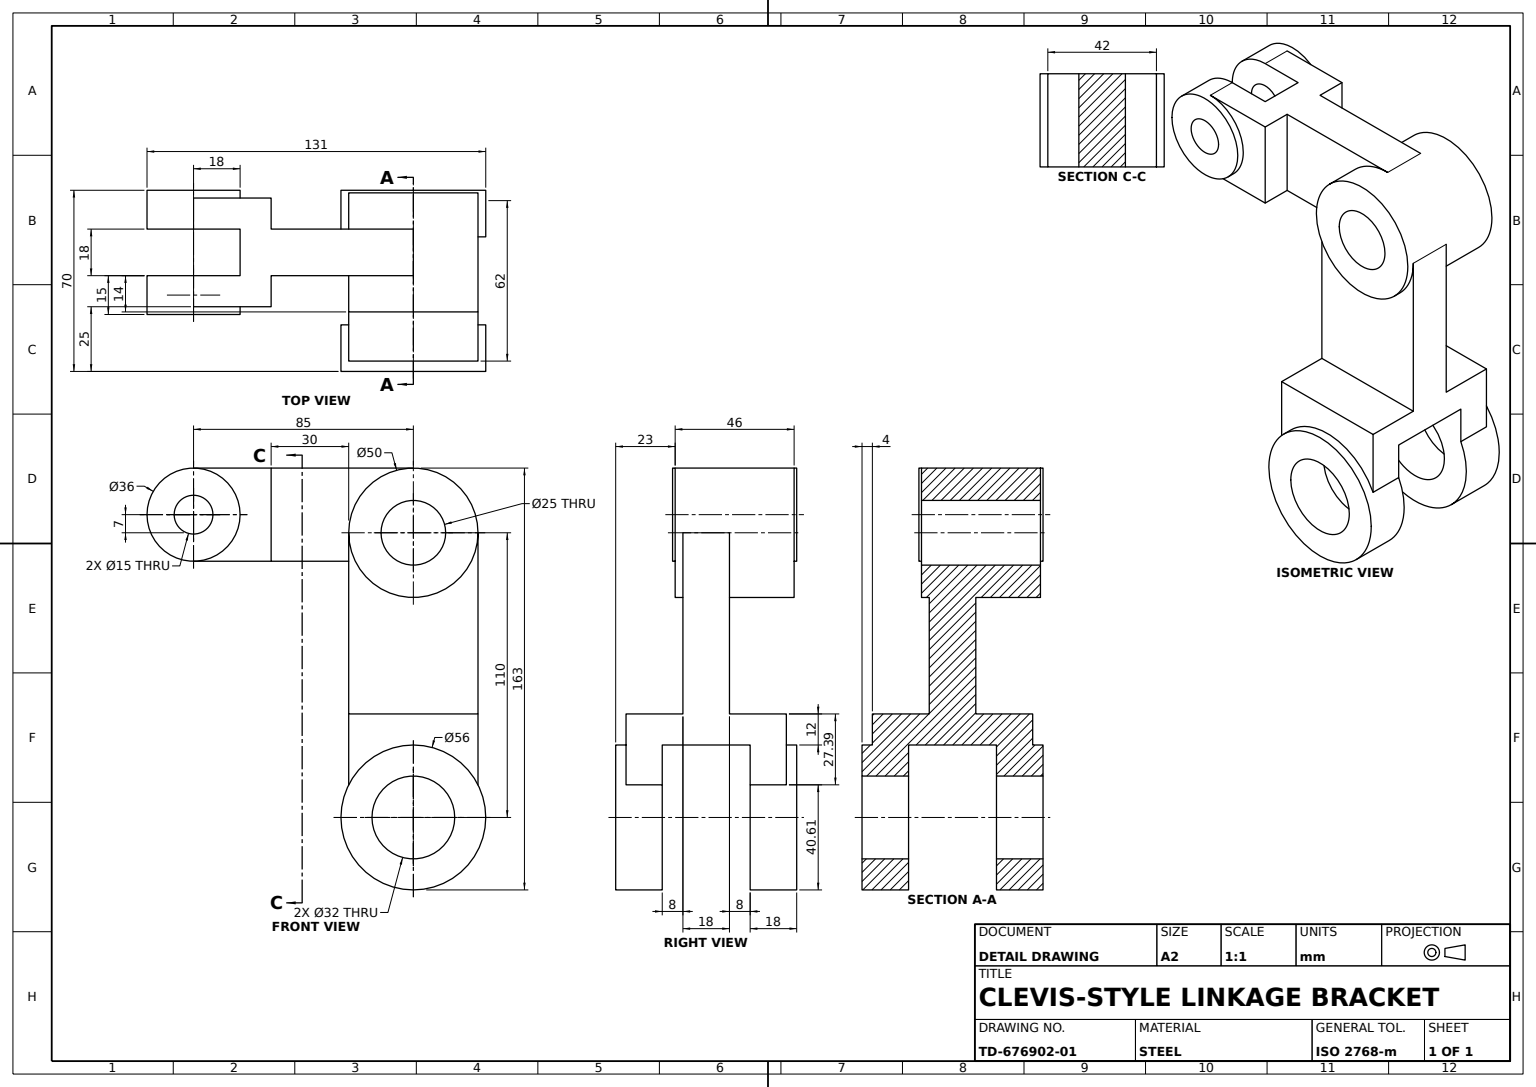
from build123d import *

# Parameters (mm, degrees)
LOWER_HUB_A_SKETCH_R        = 28
LOWER_HUB_A_56_DEPTH        = 18
LOWER_HUB_B_SKETCH_R        = 28
LOWER_HUB_B_56_DEPTH        = 18
LOWER_FORK_BLOCK_DEPTH      = 48
LOWER_FORK_BLOCK_DEPTH_BACK = 14
LOWER_FORK_SLOT_SKETCH_W    = 34
LOWER_FORK_SLOT_SKETCH_H    = 15.390479787
LOWER_FORK_SLOT_DEPTH       = 65
VERTICAL_ARM_DEPTH          = 50
UPPER_HUB_DEPTH             = 3
UPPER_HUB_DEPTH_BACK        = 43
UPPER_HUB_SKETCH_R          = 25
UPPER_FORK_ARM_DEPTH        = 36
FORK_EYE_A_SKETCH_R         = 18
FORK_EYE_A_36_DEPTH         = 15
FORK_START                  = -15
FORK_EYE_B_SKETCH_R         = 18
FORK_EYE_B_DEPTH            = 15
LOWER_PIVOT_BORE_SKETCH_R   = 16
LOWER_PIVOT_BORE_32_DEPTH   = 132
UPPER_HUB_BORE_SKETCH_R     = 12.5
UPPER_HUB_BORE_25_DEPTH     = 132
FORK_EYE_BORE_SKETCH_R      = 7.5
FORK_EYE_BORE_15_DEPTH      = 132


with BuildPart() as part:
    # Lower Hub A Sketch → Lower Hub A Ø56 (new body)
    with BuildSketch(Plane(origin=(0, 0, 0), x_dir=(0, 0, -1), z_dir=(1, 0, 0))):
        Circle(LOWER_HUB_A_SKETCH_R)
    extrude(amount=-LOWER_HUB_A_56_DEPTH)



with BuildPart() as body_2:
    # Lower Hub B Sketch → Lower Hub B Ø56 (new body)
    with BuildSketch(Plane.ZY.offset(52)):
        with Locations(Location((0, 0, 0), (0, 0, 180))):
            Circle(LOWER_HUB_B_SKETCH_R)
    extrude(amount=LOWER_HUB_B_56_DEPTH)


with BuildPart() as part_1:
    add(part.part)

    add(body_2.part)  # Lower Fork Block merges body 2
    # Lower Fork Block Sketch → Lower Fork Block (add, two sides: drawn at the far end of the back side and taken through both)
    with BuildSketch(Plane.ZY.offset(18).offset(-LOWER_FORK_BLOCK_DEPTH_BACK)):
        with BuildLine():
            Line((0, 40), (25, 40))
            Line((25, 40), (25, 12.609520213))
            ThreePointArc((25, 12.609520213), (0, 28), (-25, 12.609520213))
            Line((-25, 12.609520213), (-25, 40))
            Line((-25, 40), (0, 40))
        make_face()
    extrude(amount=LOWER_FORK_BLOCK_DEPTH + LOWER_FORK_BLOCK_DEPTH_BACK)

    # Lower Fork Slot Sketch → Lower Fork Slot (cut)
    with BuildSketch(Plane.XY.offset(25)):
        with Locations((-35, 20.304760107)):
            Rectangle(LOWER_FORK_SLOT_SKETCH_W, LOWER_FORK_SLOT_SKETCH_H)
    extrude(amount=-LOWER_FORK_SLOT_DEPTH, mode=Mode.SUBTRACT)

    # Vertical Arm Sketch → Vertical Arm (add)
    with BuildSketch(Plane.XY.offset(25)):
        Polygon((-35, 40), (-26, 40), (-26, 110), (-44, 110), (-44, 40), align=None)
    extrude(amount=-VERTICAL_ARM_DEPTH)

    # Upper Hub Sketch → Upper Hub (add, two sides: drawn at the far end of the back side and taken through both)
    with BuildSketch(Plane(origin=(-26, 0, 0), x_dir=(0, 0, -1), z_dir=(1, 0, 0)).offset(-UPPER_HUB_DEPTH_BACK)):
        with Locations((0, 110)):
            Circle(UPPER_HUB_SKETCH_R)
    extrude(amount=UPPER_HUB_DEPTH + UPPER_HUB_DEPTH_BACK)

    # Upper Fork Arm Sketch → Upper Fork Arm (add)
    with BuildSketch(Plane(origin=(0, 135, 0), x_dir=(1, 0, 0), z_dir=(0, 1, 0))):
        Polygon((-37, 0), (-37, -55), (-25, -55), (-25, -85), (-37, -85), (-37, -67), (-55, -67), (-55, -85), (-67, -85), (-67, -55), (-55, -55), (-55, 0), align=None)
    extrude(amount=-UPPER_FORK_ARM_DEPTH)

    # Fork Eye A Sketch → Fork Eye A Ø36 (add)
    with BuildSketch(Plane(origin=(-55, 0, 0), x_dir=(0, 0, -1), z_dir=(1, 0, 0))):
        with Locations((-85, 117)):
            Circle(FORK_EYE_A_SKETCH_R)
    extrude(amount=-FORK_EYE_A_36_DEPTH)

    # Fork Eye B Sketch → Fork Eye B (add)
    with BuildSketch(Plane.ZY.offset(37).offset(FORK_START)):
        with Locations(Location((85, 117, 0), (0, 0, 180))):
            Circle(FORK_EYE_B_SKETCH_R)
    extrude(amount=FORK_EYE_B_DEPTH)

    # Lower Pivot Bore Sketch → Lower Pivot Bore Ø32 (cut)
    with BuildSketch(Plane(origin=(0, 0, 0), x_dir=(0, 0, -1), z_dir=(1, 0, 0))):
        with Locations(Location((0, 0, 0), (0, 0, 180))):
            Circle(LOWER_PIVOT_BORE_SKETCH_R)
    extrude(amount=-LOWER_PIVOT_BORE_32_DEPTH, mode=Mode.SUBTRACT)

    # Upper Hub Bore Sketch → Upper Hub Bore Ø25 (cut)
    with BuildSketch(Plane.ZY.offset(69)):
        with Locations((0, 110)):
            Circle(UPPER_HUB_BORE_SKETCH_R)
    extrude(amount=-UPPER_HUB_BORE_25_DEPTH, mode=Mode.SUBTRACT)

    # Fork Eye Bore Sketch → Fork Eye Bore Ø15 (cut)
    with BuildSketch(Plane.ZY.offset(70)):
        with Locations((85, 117)):
            Circle(FORK_EYE_BORE_SKETCH_R)
    extrude(amount=-FORK_EYE_BORE_15_DEPTH, mode=Mode.SUBTRACT)


solid = part_1.part
